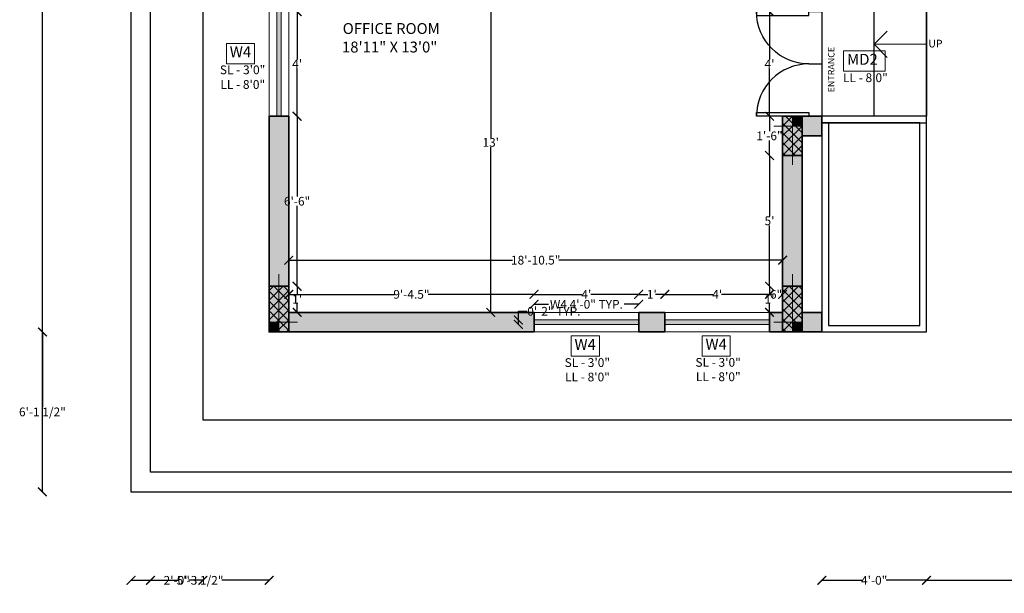
# Model space of a CAD drawing. Units: inches. Extents: x 2 to 905, y 9 to 678.
# Tile 1 of 8: x 2 to 454, y 9 to 272. Entities that reach past the tile are written whole.
import ezdxf

# ---------------------------------------------------------------- set-up
doc = ezdxf.new("R2010")
doc.units = ezdxf.units.IN
for name, color, linetype, lineweight in [('A-ANNO-DIMS', 7, 'Continuous', 18), ('A-ANNO-SYMB', 7, 'Continuous', 18), ('A-COLS', 1, 'Continuous', 35), ('A-COLS-MARK', 1, 'Continuous', 18), ('A-COLS-MARK-PATT', 3, 'Continuous', 13), ('A-COLS-PATT', 1, 'Continuous', 13), ('A-DOOR', 7, 'Continuous', 25), ('A-FLOR', 7, 'Continuous', 25), ('A-GLAZ', 4, 'Continuous', 18), ('A-WALL', 7, 'Continuous', 35), ('C-PROP', 7, 'Continuous', 25)]:
    doc.layers.add(name, color=color, linetype=linetype, lineweight=lineweight)
for name, color, linetype, lineweight, true_color in [('A-ANNO-IDEN', 251, 'Continuous', 18, 0x636466), ('A-AREA-IDEN', 252, 'Continuous', 18, 0x989898), ('A-WALL-PATT', 252, 'Continuous', 13, 0x939598)]:
    doc.layers.add(name, color=color, linetype=linetype, lineweight=lineweight, true_color=true_color)
doc.styles.add('PDF ArialMT', font='arial.ttf')
doc.styles.add('PDF Century Gothic Bold', font='txt')
doc.styles.get("Standard").update_dxf_attribs({"font": 'arial.ttf'})
doc.dimstyles.get("Standard").update_dxf_attribs({"dimtxt": 4, "dimasz": 4, "dimexe": 0.18, "dimexo": 0.0625, "dimgap": 0.09, "dimtad": 0, "dimtih": 1, "dimtoh": 1, "dimdec": 1, "dimzin": 0, "dimdsep": 46, "dimlunit": 3, "dimtxsty": 'Standard', "dimblk": 'ARCHTICK', "dimcen": 0, "dimse1": 1, "dimse2": 1, "dimclrt": 1, "dimadec": 0, "dimazin": 0, "dimtfac": 1, "dimtdec": 1, "dimtofl": 0, "dimtmove": 0, "dimatfit": 3, "dimfxl": 1, "dimtolj": 1, "dimtzin": 0, "dimarcsym": 0})
pattern_1 = [(45, (920.609, -47.8902), (-2.245064, 2.245064), []), (135, (920.609, -47.8902), (-2.245064, -2.245064), [])]

# ---------------------------------------------------------------- blocks, each defined once
blk = doc.blocks.new('*U2')
for p, q in [((0, 0), (0, -6)), ((24, 0), (24, -6))]:
    blk.add_line(p, q)
blk.add_lwpolyline([(0, 0), (0, 24), (1.75, 24), (1.75, 0)], close=True)
blk.add_arc((0, 0), 24, 0, 90)
blk = doc.blocks.new('_ArchTick')
at = {"color": 0, "linetype": 'ByBlock', "const_width": 0.15}
blk.add_lwpolyline([(-0.5, -0.5), (0.5, 0.5)], dxfattribs=at)
blk = doc.blocks.new('*D7')
at = {"layer": 'A-ANNO-DIMS', "color": 0, "lineweight": -2, "transparency": 16777216}
for p, q in [((218.07, 293.58), (218.07, 217.71)), ((218.07, 137.58), (218.07, 213.44))]:
    blk.add_line(p, q, dxfattribs=at)
at = {"layer": 'Defpoints', "color": 0, "transparency": 16777216}
for p in [(218.07, 293.58), (237.93, 293.58), (237.93, 137.58)]:
    blk.add_point(p, dxfattribs=at)
at = {"layer": 'A-ANNO-DIMS', "color": 0, "lineweight": -2, "transparency": 16777216, "xscale": 4, "yscale": 4, "zscale": 4}
for p, rotation in [((218.07, 293.58), 90), ((218.07, 137.58), 270)]:
    blk.add_blockref('_ArchTick', p, dxfattribs=dict(at, rotation=rotation))
at = {"layer": 'A-ANNO-DIMS', "color": 0, "transparency": 16777216, "insert": (218.07, 215.58), "char_height": 4, "attachment_point": 5}
blk.add_mtext("\\A1;13'", dxfattribs=at)
blk = doc.blocks.new('*D8')
at = {"layer": 'A-ANNO-DIMS', "color": 0, "lineweight": -2, "transparency": 16777216}
for p, q in [((125.43, 161.53), (228.03, 161.53)), ((351.93, 161.53), (249.34, 161.53))]:
    blk.add_line(p, q, dxfattribs=at)
at = {"layer": 'Defpoints', "color": 0, "transparency": 16777216}
for p in [(351.93, 161.53), (125.43, 139.08), (351.93, 139.08)]:
    blk.add_point(p, dxfattribs=at)
at = {"layer": 'A-ANNO-DIMS', "color": 0, "lineweight": -2, "transparency": 16777216, "xscale": 4, "yscale": 4, "zscale": 4, "rotation": 180}
blk.add_blockref('_ArchTick', (125.43, 161.53), dxfattribs=at)
at = {"layer": 'A-ANNO-DIMS', "color": 0, "lineweight": -2, "transparency": 16777216, "xscale": 4, "yscale": 4, "zscale": 4}
blk.add_blockref('_ArchTick', (351.93, 161.53), dxfattribs=at)
at = {"layer": 'A-ANNO-DIMS', "color": 0, "transparency": 16777216, "insert": (238.68, 161.53), "char_height": 4, "attachment_point": 5}
blk.add_mtext('\\A1;18\'-10.5"', dxfattribs=at)
blk = doc.blocks.new('*D13')
at = {"layer": 'A-ANNO-DIMS', "color": 0, "lineweight": -2, "transparency": 16777216}
for p, q in [((125.43, 145.85), (173.95, 145.85)), ((237.93, 145.85), (189.42, 145.85))]:
    blk.add_line(p, q, dxfattribs=at)
at = {"layer": 'Defpoints', "color": 0, "transparency": 16777216}
for p in [(237.93, 145.85), (125.43, 137.58), (237.93, 137.58)]:
    blk.add_point(p, dxfattribs=at)
at = {"layer": 'A-ANNO-DIMS', "color": 0, "lineweight": -2, "transparency": 16777216, "xscale": 4, "yscale": 4, "zscale": 4, "rotation": 180}
blk.add_blockref('_ArchTick', (125.43, 145.85), dxfattribs=at)
at = {"layer": 'A-ANNO-DIMS', "color": 0, "lineweight": -2, "transparency": 16777216, "xscale": 4, "yscale": 4, "zscale": 4}
blk.add_blockref('_ArchTick', (237.93, 145.85), dxfattribs=at)
at = {"layer": 'A-ANNO-DIMS', "color": 0, "transparency": 16777216, "insert": (181.68, 145.85), "char_height": 4, "attachment_point": 5}
blk.add_mtext('\\A1;9\'-4.5"', dxfattribs=at)
blk = doc.blocks.new('*D14')
at = {"layer": 'A-ANNO-DIMS', "color": 0, "lineweight": -2, "transparency": 16777216}
for p, q in [((237.93, 145.85), (259.92, 145.85)), ((285.93, 145.85), (263.94, 145.85))]:
    blk.add_line(p, q, dxfattribs=at)
at = {"layer": 'Defpoints', "color": 0, "transparency": 16777216}
for p in [(285.93, 145.85), (237.93, 137.58), (285.93, 137.58)]:
    blk.add_point(p, dxfattribs=at)
at = {"layer": 'A-ANNO-DIMS', "color": 0, "lineweight": -2, "transparency": 16777216, "xscale": 4, "yscale": 4, "zscale": 4, "rotation": 180}
blk.add_blockref('_ArchTick', (237.93, 145.85), dxfattribs=at)
at = {"layer": 'A-ANNO-DIMS', "color": 0, "lineweight": -2, "transparency": 16777216, "xscale": 4, "yscale": 4, "zscale": 4}
blk.add_blockref('_ArchTick', (285.93, 145.85), dxfattribs=at)
at = {"layer": 'A-ANNO-DIMS', "color": 0, "transparency": 16777216, "insert": (261.93, 145.85), "char_height": 4, "attachment_point": 5}
blk.add_mtext("\\A1;4'", dxfattribs=at)
blk = doc.blocks.new('*D15')
at = {"layer": 'A-ANNO-DIMS', "color": 0, "lineweight": -2, "transparency": 16777216}
for p, q in [((285.93, 145.85), (290.19, 145.85)), ((297.93, 145.85), (293.68, 145.85))]:
    blk.add_line(p, q, dxfattribs=at)
at = {"layer": 'Defpoints', "color": 0, "transparency": 16777216}
for p in [(297.93, 145.85), (285.93, 137.58), (297.93, 137.58)]:
    blk.add_point(p, dxfattribs=at)
at = {"layer": 'A-ANNO-DIMS', "color": 0, "lineweight": -2, "transparency": 16777216, "xscale": 4, "yscale": 4, "zscale": 4, "rotation": 180}
blk.add_blockref('_ArchTick', (285.93, 145.85), dxfattribs=at)
at = {"layer": 'A-ANNO-DIMS', "color": 0, "lineweight": -2, "transparency": 16777216, "xscale": 4, "yscale": 4, "zscale": 4}
blk.add_blockref('_ArchTick', (297.93, 145.85), dxfattribs=at)
at = {"layer": 'A-ANNO-DIMS', "color": 0, "transparency": 16777216, "insert": (291.93, 145.85), "char_height": 4, "attachment_point": 5}
blk.add_mtext("\\A1;1'", dxfattribs=at)
blk = doc.blocks.new('*D16')
at = {"layer": 'A-ANNO-DIMS', "color": 0, "lineweight": -2, "transparency": 16777216}
for p, q in [((297.93, 145.85), (319.92, 145.85)), ((345.93, 145.85), (323.94, 145.85))]:
    blk.add_line(p, q, dxfattribs=at)
at = {"layer": 'Defpoints', "color": 0, "transparency": 16777216}
for p in [(345.93, 145.85), (297.93, 137.58), (345.93, 137.58)]:
    blk.add_point(p, dxfattribs=at)
at = {"layer": 'A-ANNO-DIMS', "color": 0, "lineweight": -2, "transparency": 16777216, "xscale": 4, "yscale": 4, "zscale": 4, "rotation": 180}
blk.add_blockref('_ArchTick', (297.93, 145.85), dxfattribs=at)
at = {"layer": 'A-ANNO-DIMS', "color": 0, "lineweight": -2, "transparency": 16777216, "xscale": 4, "yscale": 4, "zscale": 4}
blk.add_blockref('_ArchTick', (345.93, 145.85), dxfattribs=at)
at = {"layer": 'A-ANNO-DIMS', "color": 0, "transparency": 16777216, "insert": (321.93, 145.85), "char_height": 4, "attachment_point": 5}
blk.add_mtext("\\A1;4'", dxfattribs=at)
blk = doc.blocks.new('*D17')
at = {"layer": 'A-ANNO-DIMS', "color": 0, "lineweight": -2, "transparency": 16777216}
for p, q in [((345.93, 145.85), (346.53, 145.85)), ((351.93, 145.85), (351.33, 145.85))]:
    blk.add_line(p, q, dxfattribs=at)
at = {"layer": 'Defpoints', "color": 0, "transparency": 16777216}
for p in [(351.93, 145.85), (345.93, 137.58), (351.93, 137.58)]:
    blk.add_point(p, dxfattribs=at)
at = {"layer": 'A-ANNO-DIMS', "color": 0, "lineweight": -2, "transparency": 16777216, "xscale": 4, "yscale": 4, "zscale": 4, "rotation": 180}
blk.add_blockref('_ArchTick', (345.93, 145.85), dxfattribs=at)
at = {"layer": 'A-ANNO-DIMS', "color": 0, "lineweight": -2, "transparency": 16777216, "xscale": 4, "yscale": 4, "zscale": 4}
blk.add_blockref('_ArchTick', (351.93, 145.85), dxfattribs=at)
at = {"layer": 'A-ANNO-DIMS', "color": 0, "transparency": 16777216, "insert": (348.93, 145.85), "char_height": 4, "attachment_point": 5}
blk.add_mtext('\\A1;6"', dxfattribs=at)
blk = doc.blocks.new('*D18')
at = {"layer": 'A-ANNO-DIMS', "color": 0, "lineweight": -2, "transparency": 16777216}
for p, q in [((345.92, 149.58), (345.92, 145.68)), ((345.92, 137.58), (345.92, 141.48))]:
    blk.add_line(p, q, dxfattribs=at)
at = {"layer": 'Defpoints', "color": 0, "transparency": 16777216}
for p in [(345.92, 149.58), (351.93, 149.58), (351.93, 137.58)]:
    blk.add_point(p, dxfattribs=at)
at = {"layer": 'A-ANNO-DIMS', "color": 0, "lineweight": -2, "transparency": 16777216, "xscale": 4, "yscale": 4, "zscale": 4}
for p, rotation in [((345.92, 149.58), 90), ((345.92, 137.58), 270)]:
    blk.add_blockref('_ArchTick', p, dxfattribs=dict(at, rotation=rotation))
at = {"layer": 'A-ANNO-DIMS', "color": 0, "transparency": 16777216, "insert": (345.92, 143.58), "char_height": 4, "attachment_point": 5}
blk.add_mtext("\\A1;1'", dxfattribs=at)
blk = doc.blocks.new('*D19')
at = {"layer": 'A-ANNO-DIMS', "color": 0, "lineweight": -2, "transparency": 16777216}
for p, q in [((345.92, 209.58), (345.92, 181.7)), ((345.92, 149.58), (345.92, 177.45))]:
    blk.add_line(p, q, dxfattribs=at)
at = {"layer": 'Defpoints', "color": 0, "transparency": 16777216}
for p in [(345.92, 209.58), (351.93, 209.58), (351.93, 149.58)]:
    blk.add_point(p, dxfattribs=at)
at = {"layer": 'A-ANNO-DIMS', "color": 0, "lineweight": -2, "transparency": 16777216, "xscale": 4, "yscale": 4, "zscale": 4}
for p, rotation in [((345.92, 209.58), 90), ((345.92, 149.58), 270)]:
    blk.add_blockref('_ArchTick', p, dxfattribs=dict(at, rotation=rotation))
at = {"layer": 'A-ANNO-DIMS', "color": 0, "transparency": 16777216, "insert": (345.92, 179.58), "char_height": 4, "attachment_point": 5}
blk.add_mtext("\\A1;5'", dxfattribs=at)
blk = doc.blocks.new('*D20')
at = {"layer": 'A-ANNO-DIMS', "color": 0, "lineweight": -2, "transparency": 16777216}
for p, q in [((345.92, 227.58), (345.92, 220.71)), ((345.92, 209.58), (345.92, 216.45))]:
    blk.add_line(p, q, dxfattribs=at)
at = {"layer": 'Defpoints', "color": 0, "transparency": 16777216}
for p in [(345.92, 227.58), (351.93, 227.58), (351.93, 209.58)]:
    blk.add_point(p, dxfattribs=at)
at = {"layer": 'A-ANNO-DIMS', "color": 0, "lineweight": -2, "transparency": 16777216, "xscale": 4, "yscale": 4, "zscale": 4}
for p, rotation in [((345.92, 227.58), 90), ((345.92, 209.58), 270)]:
    blk.add_blockref('_ArchTick', p, dxfattribs=dict(at, rotation=rotation))
at = {"layer": 'A-ANNO-DIMS', "color": 0, "transparency": 16777216, "insert": (345.92, 218.58), "char_height": 4, "attachment_point": 5}
blk.add_mtext('\\A1;1\'-6"', dxfattribs=at)
blk = doc.blocks.new('*D21')
at = {"layer": 'A-ANNO-DIMS', "color": 0, "lineweight": -2, "transparency": 16777216}
for p, q in [((345.92, 275.58), (345.92, 253.67)), ((345.92, 227.58), (345.92, 249.49))]:
    blk.add_line(p, q, dxfattribs=at)
at = {"layer": 'Defpoints', "color": 0, "transparency": 16777216}
for p in [(345.92, 275.58), (360.93, 275.58), (351.93, 227.58)]:
    blk.add_point(p, dxfattribs=at)
at = {"layer": 'A-ANNO-DIMS', "color": 0, "lineweight": -2, "transparency": 16777216, "xscale": 4, "yscale": 4, "zscale": 4}
for p, rotation in [((345.92, 275.58), 90), ((345.92, 227.58), 270)]:
    blk.add_blockref('_ArchTick', p, dxfattribs=dict(at, rotation=rotation))
at = {"layer": 'A-ANNO-DIMS', "color": 0, "transparency": 16777216, "insert": (345.92, 251.58), "char_height": 4, "attachment_point": 5}
blk.add_mtext("\\A1;4'", dxfattribs=at)
blk = doc.blocks.new('*D23')
at = {"layer": 'A-ANNO-DIMS', "color": 0, "lineweight": -2, "transparency": 16777216}
for p, q in [((129.26, 149.58), (129.26, 145.68)), ((129.26, 137.58), (129.26, 141.48))]:
    blk.add_line(p, q, dxfattribs=at)
at = {"layer": 'Defpoints', "color": 0, "transparency": 16777216}
for p in [(125.43, 149.58), (129.26, 149.58), (125.43, 137.58)]:
    blk.add_point(p, dxfattribs=at)
at = {"layer": 'A-ANNO-DIMS', "color": 0, "lineweight": -2, "transparency": 16777216, "xscale": 4, "yscale": 4, "zscale": 4}
for p, rotation in [((129.26, 149.58), 90), ((129.26, 137.58), 270)]:
    blk.add_blockref('_ArchTick', p, dxfattribs=dict(at, rotation=rotation))
at = {"layer": 'A-ANNO-DIMS', "color": 0, "transparency": 16777216, "insert": (129.26, 143.58), "char_height": 4, "attachment_point": 5}
blk.add_mtext("\\A1;1'", dxfattribs=at)
blk = doc.blocks.new('*D24')
at = {"layer": 'A-ANNO-DIMS', "color": 0, "lineweight": -2, "transparency": 16777216}
for p, q in [((129.26, 227.58), (129.26, 190.71)), ((129.26, 149.58), (129.26, 186.45))]:
    blk.add_line(p, q, dxfattribs=at)
at = {"layer": 'Defpoints', "color": 0, "transparency": 16777216}
for p in [(125.43, 227.58), (129.26, 227.58), (125.43, 149.58)]:
    blk.add_point(p, dxfattribs=at)
at = {"layer": 'A-ANNO-DIMS', "color": 0, "lineweight": -2, "transparency": 16777216, "xscale": 4, "yscale": 4, "zscale": 4}
for p, rotation in [((129.26, 227.58), 90), ((129.26, 149.58), 270)]:
    blk.add_blockref('_ArchTick', p, dxfattribs=dict(at, rotation=rotation))
at = {"layer": 'A-ANNO-DIMS', "color": 0, "transparency": 16777216, "insert": (129.26, 188.58), "char_height": 4, "attachment_point": 5}
blk.add_mtext('\\A1;6\'-6"', dxfattribs=at)
blk = doc.blocks.new('*D25')
at = {"layer": 'A-ANNO-DIMS', "color": 0, "lineweight": -2, "transparency": 16777216}
for p, q in [((129.26, 275.58), (129.26, 253.67)), ((129.26, 227.58), (129.26, 249.49))]:
    blk.add_line(p, q, dxfattribs=at)
at = {"layer": 'Defpoints', "color": 0, "transparency": 16777216}
for p in [(125.43, 275.58), (129.26, 275.58), (125.43, 227.58)]:
    blk.add_point(p, dxfattribs=at)
at = {"layer": 'A-ANNO-DIMS', "color": 0, "lineweight": -2, "transparency": 16777216, "xscale": 4, "yscale": 4, "zscale": 4}
for p, rotation in [((129.26, 275.58), 90), ((129.26, 227.58), 270)]:
    blk.add_blockref('_ArchTick', p, dxfattribs=dict(at, rotation=rotation))
at = {"layer": 'A-ANNO-DIMS', "color": 0, "transparency": 16777216, "insert": (129.26, 251.58), "char_height": 4, "attachment_point": 5}
blk.add_mtext("\\A1;4'", dxfattribs=at)
blk = doc.blocks.new('COL-DATUM-R')
h = blk.add_hatch(color=256)
h.dxf.hatch_style = 1
h.paths.add_polyline_path([(13.01, 0), (13.01, 4.5), (8.51, 4.5), (8.51, 0)])
for p, q in [((8.51, 0), (8.51, 26.48)), ((13.01, 4.5), (0, 4.5))]:
    blk.add_line(p, q)
blk.add_lwpolyline([(8.51, 0), (13.01, 0), (13.01, 4.5), (8.51, 4.5)], close=True)
blk = doc.blocks.new('COL-DATUM-L')
h = blk.add_hatch(color=256)
h.dxf.hatch_style = 1
h.paths.add_polyline_path([(4.5, 0), (4.5, 4.5), (0, 4.5), (0, 0)])
for p, q in [((4.5, 0), (4.5, 26.48)), ((0, 4.5), (13.01, 4.5))]:
    blk.add_line(p, q)
blk.add_lwpolyline([(4.5, 0), (0, 0), (0, 4.5), (4.5, 4.5)], close=True)
blk = doc.blocks.new('GLAZ-W4-48')
h = blk.add_hatch(color=256)
h.dxf.hatch_style = 1
h.paths.add_polyline_path([(48, 0), (48, 2), (0, 2), (0, 0)])
for p, q in [((0, 2), (48, 2)), ((0, 0), (48, 0))]:
    blk.add_line(p, q)
blk = doc.blocks.new('*D96')
at = {"layer": 'A-ANNO-DIMS', "color": 0, "lineweight": -2, "transparency": 16777216}
for p, q in [((237.93, 141.28), (244.6, 141.28)), ((285.93, 141.28), (279.26, 141.28))]:
    blk.add_line(p, q, dxfattribs=at)
at = {"layer": 'Defpoints', "color": 0, "transparency": 16777216}
for p in [(285.93, 141.28), (237.93, 134.08), (285.93, 134.08)]:
    blk.add_point(p, dxfattribs=at)
at = {"layer": 'A-ANNO-DIMS', "color": 0, "lineweight": -2, "transparency": 16777216, "xscale": 4, "yscale": 4, "zscale": 4, "rotation": 180}
blk.add_blockref('_ArchTick', (237.93, 141.28), dxfattribs=at)
at = {"layer": 'A-ANNO-DIMS', "color": 0, "lineweight": -2, "transparency": 16777216, "xscale": 4, "yscale": 4, "zscale": 4}
blk.add_blockref('_ArchTick', (285.93, 141.28), dxfattribs=at)
at = {"layer": 'A-ANNO-DIMS', "color": 1, "transparency": 16777216, "insert": (261.93, 141.28), "char_height": 4, "attachment_point": 5}
blk.add_mtext('\\A1;W4 4\'-0" TYP.', dxfattribs=at)
blk = doc.blocks.new('*D97')
at = {"layer": 'A-ANNO-DIMS', "color": 0, "lineweight": -2, "transparency": 16777216}
for p, q in [((230.73, 134.08), (230.73, 138.08)), ((230.73, 138.08), (234.73, 138.08)), ((230.73, 132.08), (230.73, 134.08))]:
    blk.add_line(p, q, dxfattribs=at)
at = {"layer": 'Defpoints', "color": 0, "transparency": 16777216}
for p in [(230.73, 134.08), (237.93, 134.08), (237.93, 132.08)]:
    blk.add_point(p, dxfattribs=at)
at = {"layer": 'A-ANNO-DIMS', "color": 0, "lineweight": -2, "transparency": 16777216, "xscale": 4, "yscale": 4, "zscale": 4}
for p, rotation in [((230.73, 134.08), 90), ((230.73, 132.08), 270)]:
    blk.add_blockref('_ArchTick', p, dxfattribs=dict(at, rotation=rotation))
at = {"layer": 'A-ANNO-DIMS', "color": 1, "transparency": 16777216, "insert": (247.01, 138.08), "char_height": 4, "attachment_point": 5}
blk.add_mtext('\\A1;0\'-2" TYP.', dxfattribs=at)
blk = doc.blocks.new('*D103')
at = {"layer": 'A-ANNO-DIMS', "color": 0, "lineweight": -2, "transparency": 16777216}
for p, q in [((12.45, 631.22), (12.45, 345.35)), ((12.45, 55.22), (12.45, 341.09))]:
    blk.add_line(p, q, dxfattribs=at)
at = {"layer": 'Defpoints', "color": 0, "transparency": 16777216}
for p in [(12.45, 631.22), (53.05, 631.22), (53.05, 55.22)]:
    blk.add_point(p, dxfattribs=at)
at = {"layer": 'A-ANNO-DIMS', "color": 0, "lineweight": -2, "transparency": 16777216, "xscale": 4, "yscale": 4, "zscale": 4}
for p, rotation in [((12.45, 631.22), 90), ((12.45, 55.22), 270)]:
    blk.add_blockref('_ArchTick', p, dxfattribs=dict(at, rotation=rotation))
at = {"layer": 'A-ANNO-DIMS', "color": 1, "transparency": 16777216, "insert": (12.45, 343.22), "char_height": 4, "attachment_point": 5}
blk.add_mtext('\\A1;48\'-0"', dxfattribs=at)
blk = doc.blocks.new('*D107')
at = {"layer": 'A-ANNO-DIMS', "color": 0, "lineweight": -2, "transparency": 16777216}
for p, q in [((62.05, 14.62), (68.61, 14.62)), ((86.05, 14.62), (79.49, 14.62))]:
    blk.add_line(p, q, dxfattribs=at)
at = {"layer": 'Defpoints', "color": 0, "transparency": 16777216}
for p in [(62.05, 622.22), (86.05, 598.22), (86.05, 14.62)]:
    blk.add_point(p, dxfattribs=at)
at = {"layer": 'A-ANNO-DIMS', "color": 0, "lineweight": -2, "transparency": 16777216, "xscale": 4, "yscale": 4, "zscale": 4, "rotation": 180}
blk.add_blockref('_ArchTick', (62.05, 14.62), dxfattribs=at)
at = {"layer": 'A-ANNO-DIMS', "color": 0, "lineweight": -2, "transparency": 16777216, "xscale": 4, "yscale": 4, "zscale": 4}
blk.add_blockref('_ArchTick', (86.05, 14.62), dxfattribs=at)
at = {"layer": 'A-ANNO-DIMS', "color": 1, "transparency": 16777216, "insert": (74.05, 14.62), "char_height": 4, "attachment_point": 5}
blk.add_mtext('\\A1;2\'-0"', dxfattribs=at)
blk = doc.blocks.new('*D109')
at = {"layer": 'A-ANNO-DIMS', "color": 0, "lineweight": -2, "transparency": 16777216}
for p, q in [((53.05, 14.62), (74.68, 14.62)), ((116.43, 14.62), (94.81, 14.62))]:
    blk.add_line(p, q, dxfattribs=at)
at = {"layer": 'Defpoints', "color": 0, "transparency": 16777216}
for p in [(116.43, 128.58), (53.05, 55.22), (116.43, 14.62)]:
    blk.add_point(p, dxfattribs=at)
at = {"layer": 'A-ANNO-DIMS', "color": 0, "lineweight": -2, "transparency": 16777216, "xscale": 4, "yscale": 4, "zscale": 4, "rotation": 180}
blk.add_blockref('_ArchTick', (53.05, 14.62), dxfattribs=at)
at = {"layer": 'A-ANNO-DIMS', "color": 0, "lineweight": -2, "transparency": 16777216, "xscale": 4, "yscale": 4, "zscale": 4}
blk.add_blockref('_ArchTick', (116.43, 14.62), dxfattribs=at)
at = {"layer": 'A-ANNO-DIMS', "color": 1, "transparency": 16777216, "insert": (84.74, 14.62), "char_height": 4, "attachment_point": 5}
blk.add_mtext('\\A1;5\'-3 1/2"', dxfattribs=at)
blk = doc.blocks.new('*D110')
at = {"layer": 'A-ANNO-DIMS', "color": 0, "lineweight": -2, "transparency": 16777216}
for p, q in [((12.45, 128.58), (12.45, 94.06)), ((12.45, 55.22), (12.45, 89.74))]:
    blk.add_line(p, q, dxfattribs=at)
at = {"layer": 'Defpoints', "color": 0, "transparency": 16777216}
for p in [(12.45, 128.58), (116.43, 128.58), (53.05, 55.22)]:
    blk.add_point(p, dxfattribs=at)
at = {"layer": 'A-ANNO-DIMS', "color": 0, "lineweight": -2, "transparency": 16777216, "xscale": 4, "yscale": 4, "zscale": 4}
for p, rotation in [((12.45, 128.58), 90), ((12.45, 55.22), 270)]:
    blk.add_blockref('_ArchTick', p, dxfattribs=dict(at, rotation=rotation))
at = {"layer": 'A-ANNO-DIMS', "color": 1, "transparency": 16777216, "insert": (12.45, 91.9), "char_height": 4, "attachment_point": 5}
blk.add_mtext('\\A1;6\'-1 1/2"', dxfattribs=at)
blk = doc.blocks.new('*D112')
at = {"layer": 'A-ANNO-DIMS', "color": 0, "lineweight": -2, "transparency": 16777216}
for p, q in [((897.65, 557.58), (897.65, 345.21)), ((897.65, 128.58), (897.65, 340.94))]:
    blk.add_line(p, q, dxfattribs=at)
at = {"layer": 'Defpoints', "color": 0, "transparency": 16777216}
for p in [(417.93, 557.58), (897.65, 557.58), (417.93, 128.58)]:
    blk.add_point(p, dxfattribs=at)
at = {"layer": 'A-ANNO-DIMS', "color": 0, "lineweight": -2, "transparency": 16777216, "xscale": 4, "yscale": 4, "zscale": 4}
for p, rotation in [((897.65, 557.58), 90), ((897.65, 128.58), 270)]:
    blk.add_blockref('_ArchTick', p, dxfattribs=dict(at, rotation=rotation))
at = {"layer": 'A-ANNO-DIMS', "color": 1, "transparency": 16777216, "insert": (897.65, 343.08), "char_height": 4, "attachment_point": 5}
blk.add_mtext('\\A1;35\'-9"', dxfattribs=at)
blk = doc.blocks.new('*D113')
at = {"layer": 'A-ANNO-DIMS', "color": 0, "lineweight": -2, "transparency": 16777216}
for p, q in [((369.93, 14.62), (388.45, 14.62)), ((417.93, 14.62), (399.42, 14.62))]:
    blk.add_line(p, q, dxfattribs=at)
at = {"layer": 'Defpoints', "color": 0, "transparency": 16777216}
for p in [(369.93, 128.58), (417.93, 128.58), (417.93, 14.62)]:
    blk.add_point(p, dxfattribs=at)
at = {"layer": 'A-ANNO-DIMS', "color": 0, "lineweight": -2, "transparency": 16777216, "xscale": 4, "yscale": 4, "zscale": 4, "rotation": 180}
blk.add_blockref('_ArchTick', (369.93, 14.62), dxfattribs=at)
at = {"layer": 'A-ANNO-DIMS', "color": 0, "lineweight": -2, "transparency": 16777216, "xscale": 4, "yscale": 4, "zscale": 4}
blk.add_blockref('_ArchTick', (417.93, 14.62), dxfattribs=at)
at = {"layer": 'A-ANNO-DIMS', "color": 1, "transparency": 16777216, "insert": (393.93, 14.62), "char_height": 4, "attachment_point": 5}
blk.add_mtext('\\A1;4\'-0"', dxfattribs=at)
blk = doc.blocks.new('*D114')
at = {"layer": 'A-ANNO-DIMS', "color": 0, "lineweight": -2, "transparency": 16777216}
for p, q in [((417.93, 14.62), (474.16, 14.62)), ((543.93, 14.62), (487.71, 14.62))]:
    blk.add_line(p, q, dxfattribs=at)
at = {"layer": 'Defpoints', "color": 0, "transparency": 16777216}
for p in [(417.93, 128.58), (543.93, 128.58), (543.93, 14.62)]:
    blk.add_point(p, dxfattribs=at)
at = {"layer": 'A-ANNO-DIMS', "color": 0, "lineweight": -2, "transparency": 16777216, "xscale": 4, "yscale": 4, "zscale": 4, "rotation": 180}
blk.add_blockref('_ArchTick', (417.93, 14.62), dxfattribs=at)
at = {"layer": 'A-ANNO-DIMS', "color": 0, "lineweight": -2, "transparency": 16777216, "xscale": 4, "yscale": 4, "zscale": 4}
blk.add_blockref('_ArchTick', (543.93, 14.62), dxfattribs=at)
at = {"layer": 'A-ANNO-DIMS', "color": 1, "transparency": 16777216, "insert": (480.93, 14.62), "char_height": 4, "attachment_point": 5}
blk.add_mtext('\\A1;10\'-6"', dxfattribs=at)

msp = doc.modelspace()

# ---------------------------------------------------------------- hatches: boundary and pattern name
at = {"layer": 'A-COLS-MARK-PATT'}
h = msp.add_hatch(color=256, dxfattribs=at)
h.dxf.hatch_style = 1
h.paths.add_polyline_path([(356.43, 227.58), (356.43, 223.08), (360.93, 223.08), (360.93, 227.58)])
at = {"layer": 'A-COLS-PATT'}
h = msp.add_hatch(dxfattribs=at)
h.set_pattern_fill('ANSI37', color=256)
h.set_pattern_definition(pattern_1)
h.paths.add_polyline_path([(351.93, 223.08), (356.43, 223.08), (356.43, 227.58), (351.93, 227.58)])
h.paths.add_polyline_path([(351.93, 209.58), (356.43, 209.58), (356.43, 223.08), (351.93, 223.08)])
h.paths.add_polyline_path([(356.43, 209.58), (360.93, 209.58), (360.93, 223.08), (356.43, 223.08)])
h = msp.add_hatch(dxfattribs=at)
h.set_pattern_fill('ANSI37', color=256)
h.set_pattern_definition([(45, (967.109, -47.8902), (-2.245064, 2.245064), []), (135, (967.109, -47.8902), (-2.245064, -2.245064), [])])
h.paths.add_polyline_path([(125.43, 133.08), (120.93, 133.08), (120.93, 128.58), (125.43, 128.58)])
h.paths.add_polyline_path([(125.43, 149.58), (120.93, 149.58), (120.93, 133.08), (125.43, 133.08)])
h.paths.add_polyline_path([(120.93, 149.58), (116.43, 149.58), (116.43, 133.08), (120.93, 133.08)])
h = msp.add_hatch(dxfattribs=at)
h.set_pattern_fill('ANSI37', color=256)
h.set_pattern_definition(pattern_1)
h.paths.add_polyline_path([(351.93, 133.08), (356.43, 133.08), (356.43, 128.58), (351.93, 128.58)])
h.paths.add_polyline_path([(351.93, 149.58), (356.43, 149.58), (356.43, 133.08), (351.93, 133.08)])
h.paths.add_polyline_path([(356.43, 149.58), (360.93, 149.58), (360.93, 133.08), (356.43, 133.08)])
at = {"layer": 'A-WALL-PATT'}
h = msp.add_hatch(color=256, dxfattribs=at)
h.dxf.hatch_style = 1
h.paths.add_polyline_path([(125.43, 227.58), (116.43, 227.58), (116.43, 128.58), (237.93, 128.58), (237.93, 137.58), (125.43, 137.58)])
h.paths.add_polyline_path([(249.93, 302.58), (183.93, 302.58), (183.93, 320.58), (179.43, 320.58), (179.43, 302.58), (116.43, 302.58), (116.43, 275.58), (125.43, 275.58), (125.43, 293.58), (249.93, 293.58), (249.93, 297.58)], flags=0)
h.paths.add_polyline_path([(369.93, 137.58), (360.93, 137.58), (360.93, 218.58), (369.93, 218.58), (369.93, 227.58), (363.93, 227.58), (351.93, 227.58), (351.93, 137.58), (345.93, 137.58), (345.93, 128.58), (360.93, 128.58), (369.93, 128.58)])
h.paths.add_polyline_path([(297.93, 137.58), (285.93, 137.58), (285.93, 128.58), (297.93, 128.58)])
h.paths.add_polyline_path([(369.93, 444.58), (360.93, 444.58), (360.93, 371.58), (183.93, 371.58), (183.93, 460.08), (125.43, 460.08), (125.43, 466.08), (116.43, 466.08), (116.43, 449.58), (120.43, 449.58), (125.43, 449.58), (125.43, 455.58), (179.43, 455.58), (179.43, 371.58), (125.43, 371.58), (125.43, 389.58), (116.43, 389.58), (116.43, 362.58), (179.43, 362.58), (179.43, 344.58), (183.93, 344.58), (183.93, 362.58), (291.93, 362.58), (291.93, 302.58), (285.93, 302.58), (285.93, 293.58), (309.93, 293.58), (309.93, 302.58), (300.93, 302.58), (300.93, 362.58), (360.93, 362.58), (360.93, 302.58), (351.93, 302.58), (351.93, 293.58), (360.93, 293.58), (360.93, 275.58), (363.93, 275.58), (369.93, 275.58)])
h.paths.add_polyline_path([(282.93, 557.58), (116.43, 557.58), (116.43, 506.08), (120.43, 506.08), (125.43, 506.08), (125.43, 548.58), (282.93, 548.58)])
h.paths.add_polyline_path([(369.93, 557.58), (330.93, 557.58), (330.93, 548.58), (360.93, 548.58), (360.93, 504.58), (369.93, 504.58)])

# ---------------------------------------------------------------- linework, layer by layer
at = {"layer": 'A-ANNO-IDEN'}
for points in [[(96.92, 261.02), (109.71, 261.02), (109.71, 251.65), (96.92, 251.65)], [(379.93, 257.6), (399.01, 257.6), (399.01, 248.23), (379.93, 248.23)], [(255.02, 126.78), (267.92, 126.78), (267.92, 117.41), (255.02, 117.41)], [(314.99, 126.88), (327.89, 126.88), (327.89, 117.51), (314.99, 117.51)]]:
    msp.add_lwpolyline(points, close=True, dxfattribs=at)
at = {"layer": 'A-ANNO-SYMB'}
msp.add_line((393.93, 260.58), (417.93, 260.58), dxfattribs=at)
msp.add_lwpolyline([(399.94, 266.59), (393.93, 260.58), (399.94, 254.57)], dxfattribs=at)
at = {"layer": 'A-COLS'}
for points in [[(360.93, 209.58), (351.93, 209.58), (351.93, 227.58), (360.93, 227.58)], [(116.43, 149.58), (125.43, 149.58), (125.43, 128.58), (116.43, 128.58)], [(360.93, 149.58), (351.93, 149.58), (351.93, 128.58), (360.93, 128.58)]]:
    msp.add_lwpolyline(points, close=True, dxfattribs=at)
at = {"layer": 'A-COLS-MARK'}
for p, q in [((356.43, 227.58), (356.43, 205.31)), ((360.93, 223.08), (347.92, 223.08))]:
    msp.add_line(p, q, dxfattribs=at)
msp.add_lwpolyline([(356.43, 227.58), (360.93, 227.58), (360.93, 223.08), (356.43, 223.08)], close=True, dxfattribs=at)
at = {"layer": 'A-FLOR'}
msp.add_line((372.93, 224.58), (369.93, 224.58), dxfattribs=at)
for points in [[(369.93, 224.58), (417.93, 224.58), (417.93, 371.58), (369.93, 371.58)], [(417.93, 227.58), (393.93, 227.58), (393.93, 293.58), (417.93, 293.58)], [(369.93, 128.58), (417.93, 128.58), (417.93, 227.58), (369.93, 227.58)], [(372.93, 131.58), (414.93, 131.58), (414.93, 224.58), (372.93, 224.58)]]:
    msp.add_lwpolyline(points, close=True, dxfattribs=at)
at = {"layer": 'A-GLAZ'}
for points in [[(116.43, 227.58), (116.43, 275.58), (125.43, 275.58), (125.43, 227.58)], [(237.93, 137.58), (285.93, 137.58), (285.93, 128.58), (237.93, 128.58)], [(297.93, 137.58), (345.93, 137.58), (345.93, 128.58), (297.93, 128.58)]]:
    msp.add_lwpolyline(points, close=True, dxfattribs=at)
at = {"layer": 'A-WALL'}
for p, q in [((125.43, 227.58), (116.43, 227.58)), ((116.43, 227.58), (116.43, 128.58)), ((116.43, 227.58), (125.43, 227.58)), ((125.43, 227.58), (125.43, 137.58)), ((360.93, 218.58), (360.93, 137.58)), ((360.93, 218.58), (360.93, 137.58)), ((125.43, 137.58), (237.93, 137.58)), ((237.93, 137.58), (237.93, 128.58)), ((285.93, 137.58), (285.93, 128.58)), ((285.93, 137.58), (297.93, 137.58)), ((297.93, 137.58), (297.93, 128.58)), ((297.93, 137.58), (297.93, 128.58)), ((345.93, 137.58), (345.93, 128.58)), ((345.93, 137.58), (345.93, 128.58)), ((369.93, 137.58), (360.93, 137.58)), ((369.93, 128.58), (369.93, 137.58)), ((116.43, 128.58), (237.93, 128.58)), ((285.93, 128.58), (297.93, 128.58)), ((345.93, 128.58), (360.93, 128.58)), ((360.93, 128.58), (369.93, 128.58))]:
    msp.add_line(p, q, dxfattribs=at)
msp.add_lwpolyline([(345.93, 137.58), (351.93, 137.58), (351.93, 227.58), (369.93, 227.58), (369.93, 218.58), (360.93, 218.58)], dxfattribs=at)
at = {"layer": 'C-PROP'}
msp.add_lwpolyline([(857.05, 535.22), (857.05, 631.22), (53.05, 631.22), (53.05, 55.22), (857.05, 55.22), (857.05, 355.22), (848.05, 355.22), (848.05, 64.22), (62.05, 64.22), (62.05, 622.22), (848.05, 622.22), (848.05, 535.22)], close=True, dxfattribs=at)
msp.add_lwpolyline([(848.05, 598.22), (86.05, 598.22), (86.05, 88.22), (824.05, 88.22), (824.05, 355.22), (836.05, 355.22), (848.05, 355.22)], dxfattribs=at)

# ---------------------------------------------------------------- block references
at = {"layer": 'A-COLS-MARK'}
for name, p in [('COL-DATUM-L', (116.43, 128.58)), ('COL-DATUM-R', (347.92, 128.58))]:
    msp.add_blockref(name, p, dxfattribs=at)
at = {"layer": 'A-DOOR', "xscale": -1, "rotation": 90}
msp.add_blockref('*U2', (363.93, 275.58), dxfattribs=at)
at = {"layer": 'A-DOOR', "rotation": 90}
msp.add_blockref('*U2', (363.93, 227.58), dxfattribs=at)
at = {"layer": 'A-GLAZ', "rotation": 90.00000000000003}
msp.add_blockref('GLAZ-W4-48', (121.93, 227.58), dxfattribs=at)
at = {"layer": 'A-GLAZ'}
msp.add_blockref('GLAZ-W4-48', (237.93, 132.08), dxfattribs=at)
at = {"layer": 'A-GLAZ', "extrusion": (0, 0, -1), "zscale": -1, "rotation": 180}
msp.add_blockref('GLAZ-W4-48', (-297.93, 134.08), dxfattribs=at)

# ---------------------------------------------------------------- texts
at = {"layer": 'A-ANNO-IDEN', "attachment_point": 4, "style": 'PDF ArialMT'}
for s, insert, char_height in [('W4', (98.36, 256.47), 5.029), ('MD2', (381.5, 253.05), 5.029), ('SL - 3\'0"', (93.84, 248.37), 4.023), ('LL - 8\'0"', (94.06, 241.64), 4.023), ('LL - 8\'0"', (379.62, 244.73), 4.023), ('W4', (256.47, 122.23), 5.029), ('W4', (316.56, 122.33), 5.029), ('SL - 3\'0"', (251.95, 114.01), 4.023), ('SL - 3\'0"', (311.93, 114.11), 4.023), ('LL - 8\'0"', (252.17, 107.39), 4.023), ('LL - 8\'0"', (312.15, 107.5), 4.023)]:
    msp.add_mtext(s, dxfattribs=dict(at, insert=insert, char_height=char_height))
at = {"layer": 'A-ANNO-SYMB', "insert": (418.77, 260.46), "char_height": 3.52, "attachment_point": 4, "style": 'PDF ArialMT'}
msp.add_mtext('UP', dxfattribs=at)
at = {"layer": 'A-AREA-IDEN', "char_height": 5, "attachment_point": 4, "style": 'PDF Century Gothic Bold'}
for s, insert in [('OFFICE ROOM', (150.18, 267.18)), ('18\'11" X 13\'0"', (149.85, 258.69))]:
    msp.add_mtext(s, dxfattribs=dict(at, insert=insert))
at = {"layer": 'A-AREA-IDEN', "insert": (374.61, 238.54), "char_height": 3, "attachment_point": 4, "rotation": 90, "style": 'PDF Century Gothic Bold'}
msp.add_mtext('ENTRANCE', dxfattribs=at)

# ---------------------------------------------------------------- dimensions: what is measured, and where the dimension line sits
at = {"layer": 'A-ANNO-DIMS'}
for base, p1, p2, override, picture, middle in [((12.45, 631.22), (53.05, 55.22), (53.05, 631.22), {"dimdec": 1, "dimlfac": 1, "dimrnd": 0, "dimzin": 1, "dimdsep": 46, "dimlunit": 4, "dimfrac": 2}, '*D103', (12.45, 343.22)), ((897.65, 557.58), (417.93, 128.58), (417.93, 557.58), {"dimdec": 1, "dimlfac": 1, "dimrnd": 0, "dimzin": 1, "dimdsep": 46, "dimlunit": 4, "dimfrac": 2}, '*D112', (897.65, 343.08)), ((218.07, 293.58), (237.93, 137.58), (237.93, 293.58), {"dimclrd": 0, "dimclre": 0, "dimclrt": 0}, '*D7', (218.07, 215.58)), ((129.26, 275.58), (125.43, 227.58), (125.43, 275.58), {"dimclrd": 0, "dimclre": 0, "dimclrt": 0, "dimtmove": 1}, '*D25', (129.26, 251.58)), ((345.92, 275.58), (351.93, 227.58), (360.93, 275.58), {"dimclrd": 0, "dimclre": 0, "dimclrt": 0, "dimtmove": 1}, '*D21', (345.92, 251.58)), ((129.26, 227.58), (125.43, 149.58), (125.43, 227.58), {"dimdec": 0, "dimclrd": 0, "dimclre": 0, "dimclrt": 0, "dimtmove": 1}, '*D24', (129.26, 188.58)), ((345.92, 227.58), (351.93, 209.58), (351.93, 227.58), {"dimdec": 0, "dimclrd": 0, "dimclre": 0, "dimclrt": 0, "dimtmove": 1}, '*D20', (345.92, 218.58)), ((345.92, 209.58), (351.93, 149.58), (351.93, 209.58), {"dimclrd": 0, "dimclre": 0, "dimclrt": 0, "dimtmove": 1}, '*D19', (345.92, 179.58)), ((129.26, 149.58), (125.43, 137.58), (125.43, 149.58), {"dimclrd": 0, "dimclre": 0, "dimclrt": 0}, '*D23', (129.26, 143.58)), ((345.92, 149.58), (351.93, 137.58), (351.93, 149.58), {"dimclrd": 0, "dimclre": 0, "dimclrt": 0}, '*D18', (345.92, 143.58)), ((12.45, 128.58), (53.05, 55.22), (116.43, 128.58), {"dimdec": 1, "dimlfac": 1, "dimrnd": 0, "dimzin": 1, "dimdsep": 46, "dimlunit": 4, "dimfrac": 2}, '*D110', (12.45, 91.9))]:
    dim = msp.add_linear_dim(base=base, p1=p1, p2=p2, angle=90, dimstyle='Standard', override=override, dxfattribs=at)
    dim.commit()
    dim.dimension.update_dxf_attribs({"geometry": picture, "text_midpoint": middle})
for base, p1, p2, override, picture, middle in [((86.05, 14.62), (62.05, 622.22), (86.05, 598.22), {"dimdec": 1, "dimlfac": 1, "dimrnd": 0, "dimzin": 1, "dimdsep": 46, "dimlunit": 4, "dimfrac": 2}, '*D107', (74.05, 14.62)), ((351.93, 161.53), (125.43, 139.08), (351.93, 139.08), {"dimclrd": 0, "dimclre": 0, "dimclrt": 0}, '*D8', (238.68, 161.53)), ((237.93, 145.85), (125.43, 137.58), (237.93, 137.58), {"dimclrd": 0, "dimclre": 0, "dimclrt": 0}, '*D13', (181.68, 145.85)), ((285.93, 145.85), (237.93, 137.58), (285.93, 137.58), {"dimclrd": 0, "dimclre": 0, "dimclrt": 0, "dimtmove": 1}, '*D14', (261.93, 145.85)), ((297.93, 145.85), (285.93, 137.58), (297.93, 137.58), {"dimclrd": 0, "dimclre": 0, "dimclrt": 0, "dimtmove": 1}, '*D15', (291.93, 145.85)), ((345.93, 145.85), (297.93, 137.58), (345.93, 137.58), {"dimclrd": 0, "dimclre": 0, "dimclrt": 0, "dimtmove": 1}, '*D16', (321.93, 145.85)), ((351.93, 145.85), (345.93, 137.58), (351.93, 137.58), {"dimdec": 0, "dimclrd": 0, "dimclre": 0, "dimclrt": 0, "dimtmove": 1}, '*D17', (348.93, 145.85)), ((116.43, 14.62), (53.05, 55.22), (116.43, 128.58), {"dimdec": 1, "dimlfac": 1, "dimrnd": 0, "dimzin": 1, "dimdsep": 46, "dimlunit": 4, "dimfrac": 2}, '*D109', (84.74, 14.62)), ((417.93, 14.62), (369.93, 128.58), (417.93, 128.58), {"dimdec": 1, "dimlfac": 1, "dimrnd": 0, "dimzin": 1, "dimdsep": 46, "dimlunit": 4, "dimfrac": 2}, '*D113', (393.93, 14.62)), ((543.93, 14.62), (417.93, 128.58), (543.93, 128.58), {"dimdec": 1, "dimlfac": 1, "dimrnd": 0, "dimzin": 1, "dimdsep": 46, "dimlunit": 4, "dimfrac": 2}, '*D114', (480.93, 14.62))]:
    dim = msp.add_linear_dim(base=base, p1=p1, p2=p2, dimstyle='Standard', override=override, dxfattribs=at)
    dim.commit()
    dim.dimension.update_dxf_attribs({"geometry": picture, "text_midpoint": middle})
dim = msp.add_linear_dim(base=(285.93, 141.28), p1=(237.93, 134.08), p2=(285.93, 134.08), text='W4 <> TYP.', dimstyle='Standard', override={"dimdec": 1, "dimlfac": 1, "dimrnd": 0, "dimzin": 1, "dimdsep": 46, "dimlunit": 4, "dimfrac": 2}, dxfattribs=at)
dim.commit()
dim.dimension.update_dxf_attribs({"geometry": '*D96', "text_midpoint": (261.93, 141.28)})
dim = msp.add_linear_dim(base=(230.73, 134.08), p1=(237.93, 132.08), p2=(237.93, 134.08), angle=90, text='<> TYP.', dimstyle='Standard', override={"dimdec": 1, "dimlfac": 1, "dimrnd": 0, "dimzin": 1, "dimdsep": 46, "dimlunit": 4, "dimfrac": 2}, dxfattribs=at)
dim.commit()
dim.dimension.update_dxf_attribs({"geometry": '*D97', "text_midpoint": (247.01, 138.08)})

doc.saveas('drawing.dxf')
